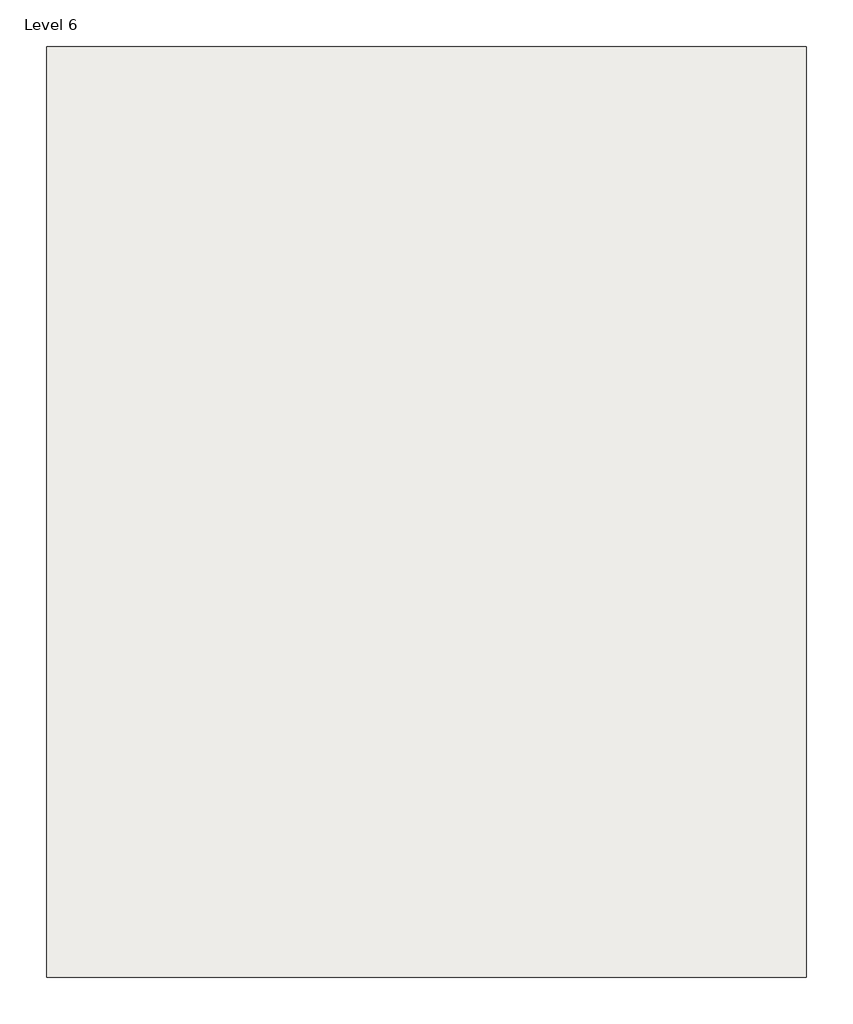
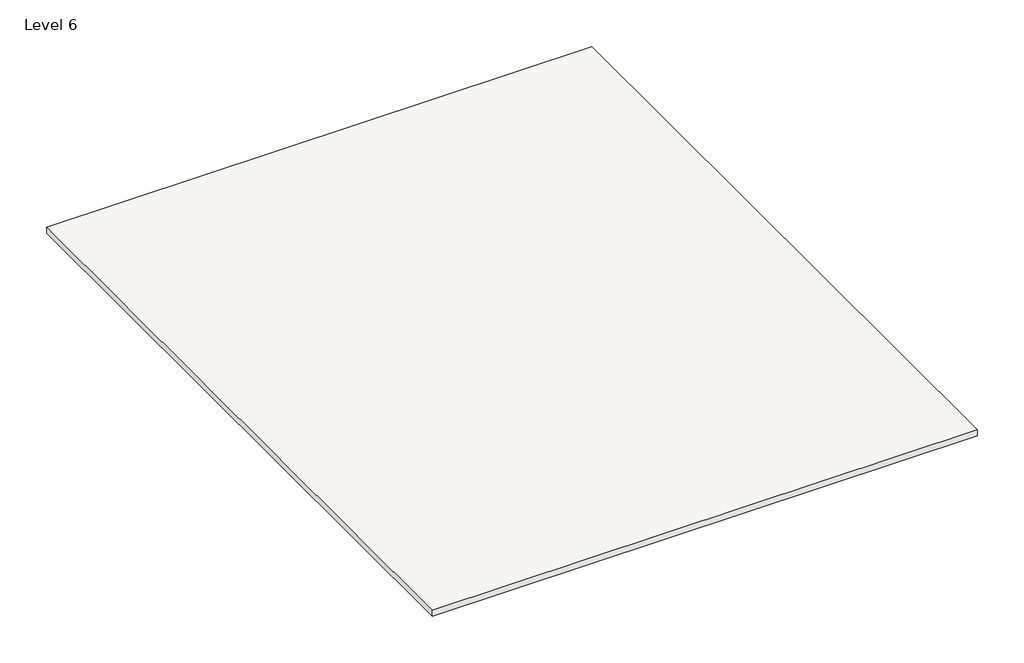
# One storey: 1 roof.
"""IFC4 building model written with IfcOpenShell, lengths in millimetres."""

from ifc_helpers import new_model, si_unit, frame, origin, place, context, project, spatial, polyline, outline, extrude, element, save

model = new_model("IFC4")

# Units and contexts
model_context = context("Model", 3, world=origin())
ifc_project = project(units=[si_unit("LENGTHUNIT", "METRE", prefix="MILLI")], contexts=[model_context])

# Site, building, storey
site = spatial("IfcSite", under=ifc_project)
building = spatial("IfcBuilding", under=site)
storey = spatial("IfcBuildingStorey", under=building, Name="Level 6", Elevation=12801.6)

# Roof
placement = place(None, origin())
element("IfcRoof", 1, ObjectType="Generic - 12\"", at=placement, inside=storey, context=model_context, shape_type="SweptSolid", body=[
    extrude(outline(polyline([(-7919.6243007, 9691.577558), (5262.9756993, 9691.577558), (5262.9756993, -6462.822442), (-7919.6243007, -6462.822442), (-7919.6243007, 9691.577558)])), frame((0.0, 0.0, 12649.2), z_axis=(0.0, 0.0, 1.0), x_axis=(1.0, 0.0, 0.0)), (0.0, 0.0, 1.0), 152.4),
])

save(model, "model.ifc")

# Revit data of these elements
# Type "Generic - 12\""
#   Assembly Code = "B1020"
#   Layers, outside or top first: 0' - 6" no material (function 1)
# Element 1 (IfcRoof, "Generic - 12\"")
#   built-in parameter 1001705 = 42 (stored number, unit not read)
#   built-in parameter 1001701 = -0.5 (stored number, unit not read)
#   built-in parameter 1001710 = 33615
#   Phase Created = New Construction
#   Materials on its faces: "Default Roof"
# Materials
#   "Default Roof": colour RGB 88 101 114, transparency 0, Cost = 0
